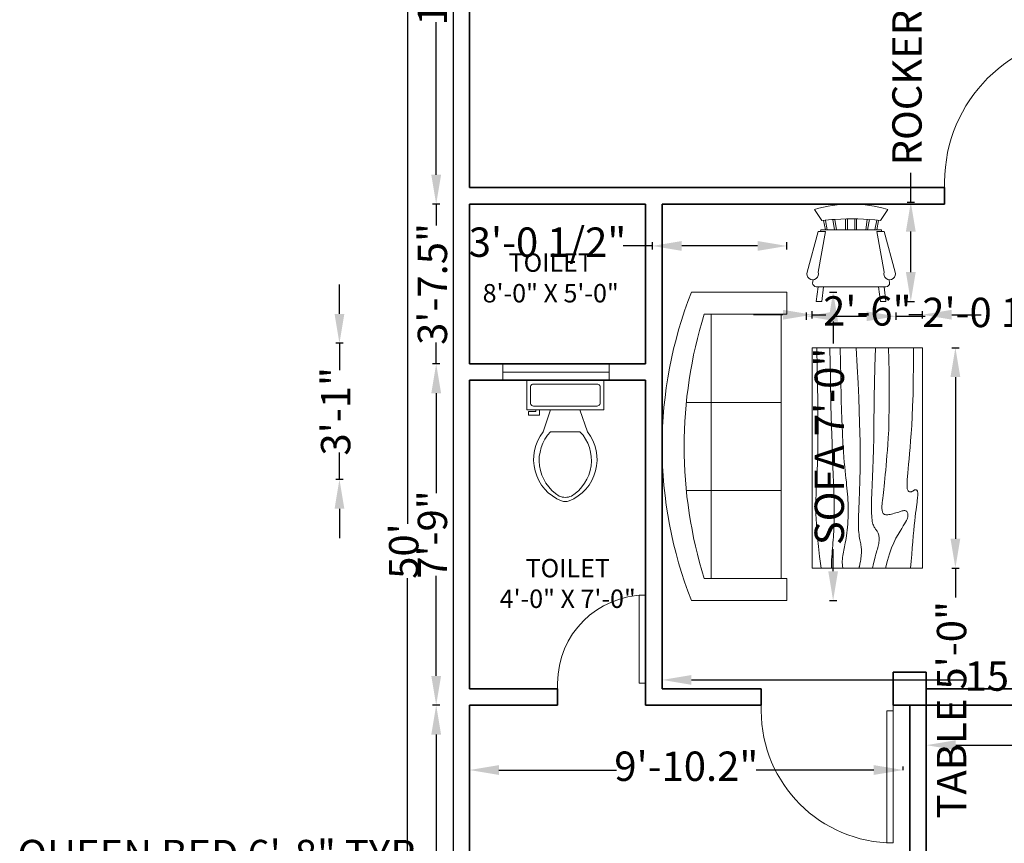
# Model space of a CAD drawing. Units: inches. Extents: x 2174 to 2692, y 577 to 1264.
# Tile 2 of 5: x 2174 to 2442, y 841 to 1065. Entities that reach past the tile are written whole.
import ezdxf

# ---------------------------------------------------------------- set-up
doc = ezdxf.new("R2010")
doc.units = ezdxf.units.IN
for name, color, linetype, lineweight in [('A-ANNO-DIMS', 2, 'Continuous', 13), ('A-AREA-IDEN', 7, 'Continuous', 18), ('A-COLS', 7, 'Continuous', 35), ('A-DOOR', 3, 'Continuous', 18), ('A-FLOR-FIXT', 9, 'Continuous', 18), ('A-FURN', 8, 'Continuous', 18), ('A-GLAZ', 4, 'Continuous', 18), ('A-WALL', 7, 'Continuous', 35), ('C-PROP', 7, 'Continuous', 25)]:
    doc.layers.add(name, color=color, linetype=linetype, lineweight=lineweight)
doc.styles.get("Standard").update_dxf_attribs({"font": 'arial.ttf'})
doc.dimstyles.new('ISO-25', dxfattribs={"dimtxt": 8, "dimasz": 8, "dimexe": 1, "dimexo": 1, "dimtad": 0, "dimdec": 1, "dimlunit": 3, "dimtxsty": 'Standard', "dimcen": 2.5, "dimclrd": 1, "dimclre": 1, "dimclrt": 1, "dimadec": 0, "dimazin": 0, "dimtfac": 1, "dimtdec": 1, "dimtmove": 0, "dimatfit": 3, "dimfxl": 1, "dimfxlon": 1, "dimarcsym": 0})

# ---------------------------------------------------------------- blocks, each defined once
blk = doc.blocks.new('Sofa - Roundback 7 ft.')
for p, q in [((-12.00002, -32.4421), (-12.00003, -6.5971)), ((11.99997, -32.4421), (11.99998, -6.5971)), ((-36.000027, -34), (-36.000027, -11.4696)), ((-35.999844, -13.3819), (35.9998, -13.3819)), ((35.99998, -34), (35.99998, -11.4696)), ((-36.000027, -32.4421), (35.99998, -32.4421))]:
    blk.add_line(p, q)
for points in [[(-36.000027, -34), (-42.000027, -34), (-42.000027, -8)], [(41.99998, -8), (41.99998, -34), (35.99998, -34)]]:
    blk.add_lwpolyline(points)
for centre, radius, start, end in [((0, -114.25), 114.25, 68.43141, 111.5686), ((-0.00001, -127.1968), 121.1968, 72.72033, 107.2797)]:
    blk.add_arc(centre, radius, start, end)
blk = doc.blocks.new('Chair - Rocking')
for p, q in [((-8, -4.5), (-10, -1.5)), ((8, -4.5), (10, -1.5)), ((-7.5, -4.5), (-7, -7)), ((-6.5, -7), (-7.02225, -4.43)), ((-4.5, -7), (-4.96674, -4.19951)), ((-4, -7), (-4.40532, -4.16272)), ((-1.5, -4.05012), (-1.5, -7)), ((-1, -7), (-1, -4.05012)), ((1, -7), (1, -4.04655)), ((1.5, -4.05012), (1.5, -7)), ((4, -7), (4.40187, -4.18694)), ((4.5, -7), (4.96761, -4.19437)), ((6.5, -7), (7, -4.4057)), ((7.5, -4.5), (7, -7)), ((-9, -7.5), (-12, -18.49999)), ((-7, -7.5), (-9, -7.5)), ((-9, -18.49999), (-7, -7.5)), ((-8.23428, -6.99939), (-8.3093, -7.47958)), ((-8.23041, -7), (8.23915, -7)), ((7, -7.5), (9, -7.5)), ((9, -18.49999), (7, -7.5)), ((8.31071, -7.48854), (8.23449, -7.00073)), ((9, -7.5), (12, -18.49999)), ((-10.36644, -20.64523), (-10.5, -21.49999)), ((10.5, -21.49999), (10.3575, -20.58798)), ((-9, -22.49999), (-9.5, -26.49999)), ((0, -22.49999), (-9.5, -22.49999)), ((-8, -26.49999), (-7.5, -22.49999)), ((0, -22.49999), (9.5, -22.49999)), ((8, -26.49999), (7.5, -22.49999)), ((9, -22.49999), (9.5, -26.49999)), ((-9.5, -26.49999), (-8, -26.49999)), ((9.5, -26.49999), (8, -26.49999))]:
    blk.add_line(p, q)
for centre, radius, start, end in [((0, -34.08333), 34.08333, 72.93847, 107.0615), ((0, -68.25004), 64.25, 93.92211, 97.15267), ((0, -68.25004), 64.25, 82.84733, 93.92211), ((-10.5, -18.99999), 1.58114, 161.5651, 18.43495), ((10.5, -18.99999), 1.58114, 161.5651, 18.43495), ((-9.5, -21.49999), 1, 180, 270), ((9.5, -21.49999), 1, 270, 0)]:
    blk.add_arc(centre, radius, start, end)
blk = doc.blocks.new('Toilet - top')
for p, q in [((9.5, -6), (9.5, -2)), ((-8, -8.5), (-8, -8)), ((-7, -8), (-7, -9.5)), ((-4, -8), (-6, -14)), ((4, -8), (6, -14)), ((-10, -8.5), (-8, -8.5)), ((-10, -9.5), (-10, -8.5)), ((-7, -9.5), (-10, -9.5)), ((4, -14), (-4, -14))]:
    blk.add_line(p, q)
blk.add_lwpolyline([(10.5, -8), (10.5, 0), (-10.5, 0), (-10.5, -8)], close=True)
for points in [[(-9.5, -2), (-9.5, -6)], [(8.5, -1), (-8.5, -1)], [(-8.5, -7), (8.5, -7)]]:
    blk.add_lwpolyline(points)
for centre, radius, start, end in [((-8.62, -1.88), 0.884, 81.8699, 188.1301), ((8.62, -1.88), 0.884, 351.8699, 98.1301), ((-8.62, -6.12), 0.884, 171.8699, 278.1301), ((8.62, -6.12), 0.884, 261.8699, 8.1301), ((3.52, -21.58), 12.17, 141.4691, 247.9714), ((4.2, -21.82), 11.33, 136.3677, 238.9468), ((-3.52, -21.58), 12.17, 292.0284, 38.5307), ((-4.2, -21.82), 11.33, 301.053, 43.6321), ((0, -27.88), 4, 245.7318, 294.2682), ((0, -29), 4, 254.8605, 285.1395)]:
    blk.add_arc(centre, radius, start, end)
blk = doc.blocks.new('Table - Rectangular Woodgrain 60 x 30 in.')
for p, q in [((0, 0), (0, -30)), ((60, 0), (0, 0)), ((60, -30), (60, 0)), ((0, -30), (60, -30))]:
    blk.add_line(p, q)
for points in [[(0, -2.4), (4.8155, -2.418), (9.0302, -2.4688), (12.709, -2.5477), (15.9167, -2.65), (18.7181, -2.7711), (21.1781, -2.9063), (23.3616, -3.0508), (25.3333, -3.2), (27.1477, -3.3495), (28.8172, -3.4958), (30.3437, -3.636), (31.7291, -3.7667), (32.9756, -3.8849), (34.0849, -3.9875), (35.059, -4.0714), (35.9, -4.1334), (36.6114, -4.1711), (37.2041, -4.1854), (37.6906, -4.1779), (38.0833, -4.15), (38.3948, -4.1034), (38.6375, -4.0396), (38.8239, -3.9602), (38.9666, -3.8667), (39.0764, -3.7608), (39.1573, -3.6448), (39.2116, -3.521), (39.2416, -3.3917), (39.2498, -3.2593), (39.2385, -3.1261), (39.21, -2.9944), (39.1666, -2.8667), (39.111, -2.7447), (39.0468, -2.6281), (38.978, -2.5163), (38.9083, -2.4083), (38.8418, -2.3035), (38.7823, -2.201), (38.7337, -2.1001), (38.7, -2), (38.6844, -1.9003), (38.6875, -1.8021), (38.7094, -1.707), (38.75, -1.6167), (38.8094, -1.5326), (38.8875, -1.4563), (38.9844, -1.3893), (39.1, -1.3333), (39.2351, -1.2896), (39.3937, -1.2583), (39.5804, -1.2396), (39.8, -1.2333), (40.057, -1.2396), (40.3562, -1.2583), (40.7023, -1.2896), (41.1, -1.3333), (41.5547, -1.3895), (42.0755, -1.4573), (42.6721, -1.5361), (43.3542, -1.625), (44.1316, -1.7233), (45.014, -1.8302), (46.0114, -1.9449), (47.1333, -2.0667), (48.3862, -2.1947), (49.7625, -2.3281), (51.2513, -2.4663), (52.8416, -2.6083), (54.5226, -2.7535), (56.2833, -2.9011), (58.1127, -3.0501), (60, -3.2)], [(0, -9.2), (6.5759, -9.0858), (11.9385, -9.0365), (16.2527, -9.0418), (19.6833, -9.0917), (22.3952, -9.1759), (24.5531, -9.2844), (26.322, -9.4069), (27.8666, -9.5333), (29.3241, -9.6553), (30.7203, -9.7719), (32.0532, -9.8837), (33.3208, -9.9917), (34.5213, -10.0965), (35.6526, -10.199), (36.7128, -10.2999), (37.7, -10.4), (38.6129, -10.4996), (39.4531, -10.5969), (40.223, -10.6895), (40.925, -10.775), (41.5613, -10.8512), (42.1344, -10.9156), (42.6465, -10.966), (43.1, -11), (43.4976, -11.0158), (43.8437, -11.0136), (44.143, -10.9942), (44.4, -10.9583), (44.6195, -10.9069), (44.8062, -10.8406), (44.9648, -10.7603), (45.1, -10.6667), (45.2155, -10.5598), (45.3114, -10.4365), (45.3871, -10.2929), (45.4416, -10.125), (45.4743, -9.929), (45.4844, -9.7011), (45.4709, -9.4371), (45.4333, -9.1333), (45.3716, -8.7883), (45.2896, -8.4104), (45.1919, -8.0107), (45.0833, -7.6), (44.9685, -7.1893), (44.8521, -6.7896), (44.7388, -6.4117), (44.6333, -6.0667), (44.54, -5.7628), (44.4614, -5.4979), (44.4001, -5.2675), (44.3583, -5.0667), (44.3384, -4.8909), (44.3427, -4.7354), (44.3736, -4.5956), (44.4333, -4.4667), (44.5236, -4.3453), (44.6427, -4.2333), (44.7884, -4.1339), (44.9583, -4.05), (45.1501, -3.9849), (45.3614, -3.9417), (45.59, -3.9234), (45.8333, -3.9333), (46.0915, -3.9749), (46.3734, -4.0531), (46.6906, -4.1736), (47.0542, -4.3417), (47.4756, -4.5629), (47.9661, -4.8427), (48.5372, -5.1866), (49.2, -5.6), (49.9676, -6.0844), (50.8594, -6.625), (51.8965, -7.2031), (53.1, -7.8), (54.491, -8.3969), (56.0906, -8.975), (57.9199, -9.5156), (60, -10)], [(0, -12.8), (5.1847, -12.9322), (9.6213, -13.0323), (13.3963, -13.1059), (16.5958, -13.1583), (19.3063, -13.1952), (21.614, -13.2219), (23.6054, -13.2439), (25.3666, -13.2667), (26.9728, -13.2947), (28.4531, -13.3281), (29.8256, -13.3663), (31.1083, -13.4083), (32.3191, -13.4535), (33.476, -13.501), (34.597, -13.5501), (35.7, -13.6), (36.7984, -13.6497), (37.8875, -13.6979), (38.9578, -13.743), (40, -13.7833), (41.0047, -13.8174), (41.9625, -13.8438), (42.864, -13.8607), (43.7, -13.8667), (44.4631, -13.8604), (45.1552, -13.8417), (45.7801, -13.8104), (46.3416, -13.7667), (46.8439, -13.7104), (47.2906, -13.6417), (47.6858, -13.5604), (48.0333, -13.4667), (48.3375, -13.3608), (48.6042, -13.2448), (48.8396, -13.121), (49.05, -12.9917), (49.2417, -12.8593), (49.4208, -12.7261), (49.5937, -12.5944), (49.7667, -12.4667), (49.9452, -12.3451), (50.1323, -12.2313), (50.3303, -12.1268), (50.5416, -12.0333), (50.7686, -11.9524), (51.0135, -11.8854), (51.2788, -11.8341), (51.5666, -11.8), (51.8785, -11.7843), (52.2116, -11.7865), (52.562, -11.8059), (52.926, -11.8417), (53.2998, -11.8931), (53.6795, -11.9594), (54.0614, -12.0397), (54.4416, -12.1333), (54.8223, -12.2401), (55.2293, -12.3625), (55.6942, -12.5037), (56.2489, -12.6667), (56.9251, -12.8547), (57.7545, -13.0708), (58.7689, -13.3182), (60, -13.6)], [(0, -18), (5.124, -17.7273), (9.6609, -17.5057), (13.6705, -17.3303), (17.2125, -17.1958), (20.3467, -17.0973), (23.1328, -17.0297), (25.6307, -16.9878), (27.9, -16.9667), (29.9928, -16.9617), (31.9302, -16.9703), (33.7254, -16.9907), (35.3917, -17.0208), (36.9423, -17.0588), (38.3906, -17.1026), (39.7499, -17.1503), (41.0333, -17.2), (42.2519, -17.2496), (43.4073, -17.2969), (44.4986, -17.3395), (45.525, -17.375), (46.4858, -17.4012), (47.3802, -17.4156), (48.2074, -17.416), (48.9667, -17.4), (49.6583, -17.3662), (50.2872, -17.3167), (50.8595, -17.2547), (51.3812, -17.1833), (51.8584, -17.1057), (52.2971, -17.025), (52.7034, -16.9443), (53.0833, -16.8667), (53.443, -16.7951), (53.789, -16.7313), (54.128, -16.6768), (54.4666, -16.6334), (54.8115, -16.6024), (55.1693, -16.5854), (55.5465, -16.5841), (55.95, -16.6), (56.3828, -16.6337), (56.8346, -16.6823), (57.2915, -16.7418), (57.7396, -16.8084), (58.165, -16.878), (58.5539, -16.9469), (58.8924, -17.0111), (59.1666, -17.0667), (59.3679, -17.1107), (59.5078, -17.1438), (59.6032, -17.1675), (59.6708, -17.1833), (59.7275, -17.193), (59.7901, -17.1979), (59.8753, -17.1998), (60, -17.2)], [(0, -22.4), (8.0098, -22.2501), (14.4094, -22.1011), (19.4168, -21.9535), (23.25, -21.8083), (26.1269, -21.6663), (28.2656, -21.5281), (29.884, -21.3947), (31.2, -21.2667), (32.3967, -21.1448), (33.5172, -21.0292), (34.5697, -20.9198), (35.5625, -20.8167), (36.5037, -20.7198), (37.4015, -20.6292), (38.2642, -20.5448), (39.1, -20.4667), (39.9164, -20.3951), (40.7187, -20.3313), (41.5117, -20.2768), (42.3, -20.2333), (43.0883, -20.2024), (43.8812, -20.1854), (44.6836, -20.1841), (45.5, -20.2), (46.3328, -20.234), (47.1747, -20.2844), (48.0163, -20.3488), (48.8479, -20.425), (49.66, -20.5106), (50.4429, -20.6031), (51.1872, -20.7004), (51.8833, -20.8), (52.5246, -20.8999), (53.1166, -20.9995), (53.6681, -21.0983), (54.1875, -21.1958), (54.6834, -21.2919), (55.1646, -21.3859), (55.6394, -21.4777), (56.1167, -21.5667), (56.6028, -21.6515), (57.0961, -21.7266), (57.5929, -21.7852), (58.0896, -21.8208), (58.5823, -21.8268), (59.0674, -21.7964), (59.5412, -21.723), (60, -21.6)], [(0, -25.2), (8.6355, -25.0504), (15.7026, -24.9031), (21.4049, -24.7606), (25.9458, -24.625), (29.529, -24.4988), (32.3578, -24.3844), (34.6359, -24.284), (36.5667, -24.2), (38.3213, -24.1341), (39.9417, -24.0854), (41.437, -24.0523), (42.8167, -24.0333), (44.0901, -24.0268), (45.2667, -24.0313), (46.3557, -24.0451), (47.3667, -24.0667), (48.309, -24.0947), (49.1928, -24.1287), (50.0284, -24.168), (50.826, -24.2125), (51.5959, -24.2617), (52.3483, -24.3151), (53.0935, -24.3725), (53.8417, -24.4334), (54.6009, -24.497), (55.3699, -24.561), (56.1454, -24.6226), (56.9239, -24.6792), (57.7021, -24.7279), (58.4764, -24.7662), (59.2435, -24.7911), (60, -24.8)], [(0, -28.8), (5.6867, -28.6681), (10.45, -28.5698), (14.407, -28.5012), (17.675, -28.4584), (20.3711, -28.4374), (22.6125, -28.4344), (24.5164, -28.4455), (26.2, -28.4667), (27.762, -28.4947), (29.2276, -28.5281), (30.6033, -28.5663), (31.8958, -28.6084), (33.1118, -28.6535), (34.2578, -28.7011), (35.3405, -28.7501), (36.3666, -28.8), (37.3443, -28.8497), (38.288, -28.8974), (39.2137, -28.9412), (40.1375, -28.9792), (41.0753, -29.0093), (42.0432, -29.0297), (43.0572, -29.0384), (44.1333, -29.0333), (45.2936, -29.0114), (46.5843, -28.9641), (48.0579, -28.8816), (49.7666, -28.7542), (51.7629, -28.5721), (54.0989, -28.3255), (56.8272, -28.0048), (60, -27.6)]]:
    blk.add_lwpolyline(points)
blk = doc.blocks.new('*D12')
at = {"layer": 'A-ANNO-DIMS', "color": 0, "lineweight": -2, "transparency": 16777216}
for p, q in [((2348.95, 885.56), (2348.95, 884.25)), ((2356.95, 885.25), (2431.92, 885.25)), ((2520.95, 885.25), (2445.99, 885.25)), ((2528.95, 885.56), (2528.95, 884.25))]:
    blk.add_line(p, q, dxfattribs=at)
at = {"layer": 'A-ANNO-DIMS', "color": 0, "transparency": 16777216}
for points in [[(2356.95, 886.58), (2356.95, 883.91), (2348.95, 885.25)], [(2520.95, 886.58), (2520.95, 883.91), (2528.95, 885.25)]]:
    blk.add_solid(points, dxfattribs=at)
at = {"layer": 'Defpoints', "color": 0, "transparency": 16777216}
for p in [(2348.95, 886.56), (2528.95, 886.56), (2348.95, 885.25)]:
    blk.add_point(p, dxfattribs=at)
at = {"layer": 'A-ANNO-DIMS', "color": 0, "transparency": 16777216, "insert": (2438.95, 885.25), "char_height": 8, "attachment_point": 5}
blk.add_mtext("15'", dxfattribs=at)
blk = doc.blocks.new('*D13')
at = {"layer": 'A-ANNO-DIMS', "color": 0, "lineweight": -2, "transparency": 16777216}
for p, q in [((2420.95, 868.48), (2420.95, 866.48)), ((2428.95, 867.48), (2479.92, 867.48)), ((2544.95, 867.48), (2493.99, 867.48)), ((2552.95, 868.48), (2552.95, 866.48))]:
    blk.add_line(p, q, dxfattribs=at)
at = {"layer": 'A-ANNO-DIMS', "color": 0, "transparency": 16777216}
for points in [[(2428.95, 868.81), (2428.95, 866.15), (2420.95, 867.48)], [(2544.95, 868.81), (2544.95, 866.15), (2552.95, 867.48)]]:
    blk.add_solid(points, dxfattribs=at)
at = {"layer": 'Defpoints', "color": 0, "transparency": 16777216}
for p in [(2420.95, 878.35), (2552.95, 878.35), (2420.95, 867.48)]:
    blk.add_point(p, dxfattribs=at)
at = {"layer": 'A-ANNO-DIMS', "color": 0, "transparency": 16777216, "insert": (2486.95, 867.48), "char_height": 8, "attachment_point": 5}
blk.add_mtext("11'", dxfattribs=at)
blk = doc.blocks.new('*D14')
at = {"layer": 'A-ANNO-DIMS', "color": 0, "lineweight": -2, "transparency": 16777216}
for p, q in [((2296.45, 860.7), (2296.45, 861.7)), ((2414.64, 860.7), (2414.64, 861.7)), ((2304.45, 860.7), (2336.52, 860.7)), ((2406.64, 860.7), (2374.57, 860.7))]:
    blk.add_line(p, q, dxfattribs=at)
at = {"layer": 'A-ANNO-DIMS', "color": 0, "transparency": 16777216}
for points in [[(2304.45, 862.03), (2304.45, 859.37), (2296.45, 860.7)], [(2406.64, 862.03), (2406.64, 859.37), (2414.64, 860.7)]]:
    blk.add_solid(points, dxfattribs=at)
at = {"layer": 'Defpoints', "color": 0, "transparency": 16777216}
for p in [(2296.45, 860.7), (2414.64, 860.7), (2414.64, 860.7)]:
    blk.add_point(p, dxfattribs=at)
at = {"layer": 'A-ANNO-DIMS', "color": 0, "transparency": 16777216, "insert": (2355.54, 860.7), "char_height": 8, "attachment_point": 5}
blk.add_mtext('9\'-10.2"', dxfattribs=at)
blk = doc.blocks.new('*U25')
for p, q in [((-24, 0), (-24, -6)), ((0, 0), (0, -6))]:
    blk.add_line(p, q)
blk.add_lwpolyline([(0, 0), (0, 24), (-1.75, 24), (-1.75, 0)], close=True)
blk.add_arc((0, 0), 24, 90, 180)
blk = doc.blocks.new('*U24')
for p, q in [((0, 0), (0, -6)), ((-40, 0), (-40, -6))]:
    blk.add_line(p, q)
blk.add_lwpolyline([(0, 0), (0, 40), (-1.75, 40), (-1.75, 0)], close=True)
blk.add_arc((0, 0), 40, 90, 180)
blk = doc.blocks.new('*U26')
for p, q in [((-36, 0), (-36, 6)), ((0, 0), (0, 6))]:
    blk.add_line(p, q)
blk.add_lwpolyline([(0, 0), (0, -36), (-1.75, -36), (-1.75, 0)], close=True)
blk.add_arc((0, 0), 36, 180, 270)
blk = doc.blocks.new('*D30')
at = {"layer": 'A-ANNO-DIMS', "color": 0, "lineweight": -2, "transparency": 16777216}
for p, q in [((2288.37, 1151.35), (2286.37, 1151.35)), ((2287.37, 1143.35), (2287.37, 1101.75)), ((2287.37, 1022.85), (2287.37, 1064.45)), ((2288.37, 1014.85), (2286.37, 1014.85))]:
    blk.add_line(p, q, dxfattribs=at)
at = {"layer": 'A-ANNO-DIMS', "color": 0, "transparency": 16777216}
for points in [[(2286.03, 1143.35), (2288.7, 1143.35), (2287.37, 1151.35)], [(2286.03, 1022.85), (2288.7, 1022.85), (2287.37, 1014.85)]]:
    blk.add_solid(points, dxfattribs=at)
at = {"layer": 'Defpoints', "color": 0, "transparency": 16777216}
for p in [(2291.95, 1151.35), (2287.37, 1014.85), (2296.45, 1014.85)]:
    blk.add_point(p, dxfattribs=at)
at = {"layer": 'A-ANNO-DIMS', "color": 0, "transparency": 16777216, "insert": (2287.37, 1083.1), "char_height": 8, "attachment_point": 5, "rotation": 90}
blk.add_mtext('11\'-4.5"', dxfattribs=at)
blk = doc.blocks.new('*D31')
at = {"layer": 'A-ANNO-DIMS', "color": 0, "lineweight": -2, "transparency": 16777216}
for p, q in [((2287.37, 1022.85), (2287.37, 1030.85)), ((2288.37, 1014.85), (2286.37, 1014.85)), ((2287.37, 1014.85), (2287.37, 1009.02)), ((2287.37, 971.35), (2287.37, 977.19)), ((2288.37, 971.35), (2286.37, 971.35)), ((2287.37, 963.35), (2287.37, 955.35))]:
    blk.add_line(p, q, dxfattribs=at)
at = {"layer": 'A-ANNO-DIMS', "color": 0, "transparency": 16777216}
for points in [[(2286.03, 1022.85), (2288.7, 1022.85), (2287.37, 1014.85)], [(2286.03, 963.35), (2288.7, 963.35), (2287.37, 971.35)]]:
    blk.add_solid(points, dxfattribs=at)
at = {"layer": 'Defpoints', "color": 0, "transparency": 16777216}
for p in [(2296.45, 1014.85), (2287.37, 971.35), (2296.45, 971.35)]:
    blk.add_point(p, dxfattribs=at)
at = {"layer": 'A-ANNO-DIMS', "color": 0, "transparency": 16777216, "insert": (2287.37, 993.1), "char_height": 8, "attachment_point": 5, "rotation": 90}
blk.add_mtext('3\'-7.5"', dxfattribs=at)
blk = doc.blocks.new('*D32')
at = {"layer": 'A-ANNO-DIMS', "color": 0, "lineweight": -2, "transparency": 16777216}
for p, q in [((2288.37, 971.35), (2286.37, 971.35)), ((2287.37, 963.35), (2287.37, 936.08)), ((2287.37, 886.35), (2287.37, 913.63)), ((2288.37, 878.35), (2286.37, 878.35))]:
    blk.add_line(p, q, dxfattribs=at)
at = {"layer": 'A-ANNO-DIMS', "color": 0, "transparency": 16777216}
for points in [[(2286.03, 963.35), (2288.7, 963.35), (2287.37, 971.35)], [(2286.03, 886.35), (2288.7, 886.35), (2287.37, 878.35)]]:
    blk.add_solid(points, dxfattribs=at)
at = {"layer": 'Defpoints', "color": 0, "transparency": 16777216}
for p in [(2296.45, 971.35), (2287.37, 878.35), (2296.45, 878.35)]:
    blk.add_point(p, dxfattribs=at)
at = {"layer": 'A-ANNO-DIMS', "color": 0, "transparency": 16777216, "insert": (2287.37, 924.85), "char_height": 8, "attachment_point": 5, "rotation": 90}
blk.add_mtext('7\'-9"', dxfattribs=at)
blk = doc.blocks.new('*D33')
at = {"layer": 'A-ANNO-DIMS', "color": 0, "lineweight": -2, "transparency": 16777216}
for p, q in [((2288.37, 878.35), (2286.37, 878.35)), ((2287.37, 870.35), (2287.37, 810.75)), ((2287.37, 713.85), (2287.37, 773.45)), ((2288.37, 705.85), (2286.37, 705.85))]:
    blk.add_line(p, q, dxfattribs=at)
at = {"layer": 'A-ANNO-DIMS', "color": 0, "transparency": 16777216}
for points in [[(2286.03, 870.35), (2288.7, 870.35), (2287.37, 878.35)], [(2286.03, 713.85), (2288.7, 713.85), (2287.37, 705.85)]]:
    blk.add_solid(points, dxfattribs=at)
at = {"layer": 'Defpoints', "color": 0, "transparency": 16777216}
for p in [(2296.45, 878.35), (2287.37, 705.85), (2296.45, 705.85)]:
    blk.add_point(p, dxfattribs=at)
at = {"layer": 'A-ANNO-DIMS', "color": 0, "transparency": 16777216, "insert": (2287.37, 792.1), "char_height": 8, "attachment_point": 5, "rotation": 90}
blk.add_mtext('14\'-4.5"', dxfattribs=at)
blk = doc.blocks.new('*D43')
at = {"layer": 'A-ANNO-DIMS', "color": 0, "lineweight": -2, "transparency": 16777216}
for p, q in [((2280.55, 1220.35), (2278.55, 1220.35)), ((2279.55, 1212.35), (2279.55, 927.77)), ((2279.55, 628.35), (2279.55, 912.94)), ((2280.55, 620.35), (2278.55, 620.35))]:
    blk.add_line(p, q, dxfattribs=at)
at = {"layer": 'A-ANNO-DIMS', "color": 0, "transparency": 16777216}
for points in [[(2278.21, 1212.35), (2280.88, 1212.35), (2279.55, 1220.35)], [(2278.21, 628.35), (2280.88, 628.35), (2279.55, 620.35)]]:
    blk.add_solid(points, dxfattribs=at)
at = {"layer": 'Defpoints', "color": 0, "transparency": 16777216}
for p in [(2291.95, 1220.35), (2279.55, 620.35), (2291.95, 620.35)]:
    blk.add_point(p, dxfattribs=at)
at = {"layer": 'A-ANNO-DIMS', "color": 0, "transparency": 16777216, "insert": (2279.55, 920.35), "char_height": 8, "attachment_point": 5, "rotation": 90}
blk.add_mtext("50'", dxfattribs=at)
blk = doc.blocks.new('*D45')
at = {"layer": 'A-ANNO-DIMS', "color": 1, "lineweight": -2, "transparency": 16777216}
for p, q in [((2296.45, 835.64), (2296.45, 837.64)), ((2376.45, 835.64), (2376.45, 837.64)), ((2296.45, 836.64), (2288.45, 836.64)), ((2368.45, 836.64), (2304.45, 836.64))]:
    blk.add_line(p, q, dxfattribs=at)
at = {"layer": 'A-ANNO-DIMS', "color": 1, "transparency": 16777216}
for points in [[(2304.45, 837.97), (2304.45, 835.3), (2296.45, 836.64)], [(2368.45, 837.97), (2368.45, 835.3), (2376.45, 836.64)]]:
    blk.add_solid(points, dxfattribs=at)
at = {"layer": 'Defpoints', "color": 0, "transparency": 16777216}
for p in [(2296.45, 836.64), (2296.45, 824.64), (2376.45, 824.64)]:
    blk.add_point(p, dxfattribs=at)
at = {"layer": 'A-ANNO-DIMS', "color": 1, "transparency": 16777216, "insert": (2228.99, 836.64), "char_height": 8, "attachment_point": 5}
blk.add_mtext('QUEEN BED 6\'-8" TYP.', dxfattribs=at)
blk = doc.blocks.new('*D51')
at = {"layer": 'A-ANNO-DIMS', "color": 1, "lineweight": -2, "transparency": 16777216}
for p, q in [((2394.55, 990.85), (2396.55, 990.85)), ((2395.55, 982.85), (2395.55, 976.86)), ((2395.55, 914.85), (2395.55, 920.85)), ((2394.55, 906.85), (2396.55, 906.85))]:
    blk.add_line(p, q, dxfattribs=at)
at = {"layer": 'A-ANNO-DIMS', "color": 1, "transparency": 16777216}
for points in [[(2394.22, 982.85), (2396.89, 982.85), (2395.55, 990.85)], [(2394.22, 914.85), (2396.89, 914.85), (2395.55, 906.85)]]:
    blk.add_solid(points, dxfattribs=at)
at = {"layer": 'Defpoints', "color": 0, "transparency": 16777216}
for p in [(2382.95, 990.85), (2395.55, 990.85), (2382.95, 906.85)]:
    blk.add_point(p, dxfattribs=at)
at = {"layer": 'A-ANNO-DIMS', "color": 1, "transparency": 16777216, "insert": (2395.55, 948.85), "char_height": 8, "attachment_point": 5, "rotation": 90}
blk.add_mtext('SOFA 7\'-0"', dxfattribs=at)
blk = doc.blocks.new('*D52')
at = {"layer": 'A-ANNO-DIMS', "color": 1, "lineweight": -2, "transparency": 16777216}
for p, q in [((2346.29, 1002.45), (2346.29, 1004.45)), ((2382.95, 1002.45), (2382.95, 1004.45)), ((2346.29, 1003.45), (2338.29, 1003.45)), ((2374.95, 1003.45), (2354.29, 1003.45))]:
    blk.add_line(p, q, dxfattribs=at)
at = {"layer": 'A-ANNO-DIMS', "color": 1, "transparency": 16777216}
for points in [[(2354.29, 1004.79), (2354.29, 1002.12), (2346.29, 1003.45)], [(2374.95, 1004.79), (2374.95, 1002.12), (2382.95, 1003.45)]]:
    blk.add_solid(points, dxfattribs=at)
at = {"layer": 'Defpoints', "color": 0, "transparency": 16777216}
for p in [(2346.29, 1003.45), (2346.29, 990.85), (2382.95, 990.85)]:
    blk.add_point(p, dxfattribs=at)
at = {"layer": 'A-ANNO-DIMS', "color": 1, "transparency": 16777216, "insert": (2317.71, 1003.45), "char_height": 8, "attachment_point": 5}
blk.add_mtext('3\'-0 1/2"', dxfattribs=at)
blk = doc.blocks.new('*D53')
at = {"layer": 'A-ANNO-DIMS', "color": 1, "lineweight": -2, "transparency": 16777216}
for p, q in [((2416.72, 1015.35), (2416.72, 1023.35)), ((2415.72, 1015.35), (2417.72, 1015.35)), ((2416.72, 996.35), (2416.72, 1007.35)), ((2415.72, 988.35), (2417.72, 988.35))]:
    blk.add_line(p, q, dxfattribs=at)
at = {"layer": 'A-ANNO-DIMS', "color": 1, "transparency": 16777216}
for points in [[(2415.39, 1007.35), (2418.06, 1007.35), (2416.72, 1015.35)], [(2415.39, 996.35), (2418.06, 996.35), (2416.72, 988.35)]]:
    blk.add_solid(points, dxfattribs=at)
at = {"layer": 'Defpoints', "color": 0, "transparency": 16777216}
for p in [(2412.67, 1015.35), (2416.72, 1015.35), (2412.67, 988.35)]:
    blk.add_point(p, dxfattribs=at)
at = {"layer": 'A-ANNO-DIMS', "color": 1, "transparency": 16777216, "insert": (2416.72, 1059.86), "char_height": 8, "attachment_point": 5, "rotation": 90}
blk.add_mtext('ROCKER 2\'-3"', dxfattribs=at)
blk = doc.blocks.new('*D54')
at = {"layer": 'A-ANNO-DIMS', "color": 1, "lineweight": -2, "transparency": 16777216}
for p, q in [((2388.24, 985.3), (2388.24, 983.3)), ((2412.67, 985.3), (2412.67, 983.3)), ((2396.24, 984.3), (2404.67, 984.3)), ((2412.67, 984.3), (2420.67, 984.3))]:
    blk.add_line(p, q, dxfattribs=at)
at = {"layer": 'A-ANNO-DIMS', "color": 1, "transparency": 16777216}
for points in [[(2396.24, 985.64), (2396.24, 982.97), (2388.24, 984.3)], [(2404.67, 985.64), (2404.67, 982.97), (2412.67, 984.3)]]:
    blk.add_solid(points, dxfattribs=at)
at = {"layer": 'Defpoints', "color": 0, "transparency": 16777216}
for p in [(2388.24, 988.35), (2412.67, 988.35), (2412.67, 984.3)]:
    blk.add_point(p, dxfattribs=at)
at = {"layer": 'A-ANNO-DIMS', "color": 1, "transparency": 16777216, "insert": (2441.32, 984.3), "char_height": 8, "attachment_point": 5}
blk.add_mtext('2\'-0 1/2"', dxfattribs=at)
blk = doc.blocks.new('*D61')
at = {"layer": 'A-ANNO-DIMS', "color": 1, "lineweight": -2, "transparency": 16777216}
for p, q in [((2427.87, 975.72), (2429.87, 975.72)), ((2428.87, 967.72), (2428.87, 923.72)), ((2427.87, 915.72), (2429.87, 915.72)), ((2428.87, 915.72), (2428.87, 907.72))]:
    blk.add_line(p, q, dxfattribs=at)
at = {"layer": 'A-ANNO-DIMS', "color": 1, "transparency": 16777216}
for points in [[(2427.54, 967.72), (2430.21, 967.72), (2428.87, 975.72)], [(2427.54, 923.72), (2430.21, 923.72), (2428.87, 915.72)]]:
    blk.add_solid(points, dxfattribs=at)
at = {"layer": 'Defpoints', "color": 0, "transparency": 16777216}
for p in [(2419.87, 975.72), (2419.87, 915.72), (2428.87, 915.72)]:
    blk.add_point(p, dxfattribs=at)
at = {"layer": 'A-ANNO-DIMS', "color": 1, "transparency": 16777216, "insert": (2428.87, 877.1), "char_height": 8, "attachment_point": 5, "rotation": 90}
blk.add_mtext('TABLE 5\'-0"', dxfattribs=at)
blk = doc.blocks.new('*D62')
at = {"layer": 'A-ANNO-DIMS', "color": 1, "lineweight": -2, "transparency": 16777216}
for p, q in [((2389.87, 983.72), (2389.87, 985.72)), ((2419.87, 983.72), (2419.87, 985.72)), ((2381.87, 984.72), (2373.87, 984.72)), ((2389.87, 984.72), (2393.55, 984.72)), ((2419.87, 984.72), (2416.2, 984.72)), ((2427.87, 984.72), (2435.87, 984.72))]:
    blk.add_line(p, q, dxfattribs=at)
at = {"layer": 'A-ANNO-DIMS', "color": 1, "transparency": 16777216}
for points in [[(2381.87, 986.05), (2381.87, 983.38), (2389.87, 984.72)], [(2427.87, 986.05), (2427.87, 983.38), (2419.87, 984.72)]]:
    blk.add_solid(points, dxfattribs=at)
at = {"layer": 'Defpoints', "color": 0, "transparency": 16777216}
for p in [(2419.87, 984.72), (2389.87, 975.72), (2419.87, 975.72)]:
    blk.add_point(p, dxfattribs=at)
at = {"layer": 'A-ANNO-DIMS', "color": 1, "transparency": 16777216, "insert": (2404.87, 984.72), "char_height": 8, "attachment_point": 5}
blk.add_mtext('2\'-6"', dxfattribs=at)
blk = doc.blocks.new('*D63')
at = {"layer": 'A-ANNO-DIMS', "color": 1, "lineweight": -2, "transparency": 16777216}
for p, q in [((2360.45, 590.4), (2360.45, 588.4)), ((2392.45, 590.4), (2392.45, 588.4)), ((2352.45, 589.4), (2344.45, 589.4)), ((2360.45, 589.4), (2365.13, 589.4)), ((2392.45, 589.4), (2387.78, 589.4)), ((2400.45, 589.4), (2408.45, 589.4))]:
    blk.add_line(p, q, dxfattribs=at)
at = {"layer": 'A-ANNO-DIMS', "color": 1, "transparency": 16777216}
for points in [[(2352.45, 590.74), (2352.45, 588.07), (2360.45, 589.4)], [(2400.45, 590.74), (2400.45, 588.07), (2392.45, 589.4)]]:
    blk.add_solid(points, dxfattribs=at)
at = {"layer": 'Defpoints', "color": 0, "transparency": 16777216}
for p in [(2360.45, 1155.85), (2392.45, 1155.6), (2392.45, 589.4)]:
    blk.add_point(p, dxfattribs=at)
at = {"layer": 'A-ANNO-DIMS', "color": 1, "transparency": 16777216, "insert": (2376.45, 589.4), "char_height": 8, "attachment_point": 5}
blk.add_mtext('2\'-8"', dxfattribs=at)
blk = doc.blocks.new('*D65')
at = {"layer": 'A-ANNO-DIMS', "color": 1, "lineweight": -2, "transparency": 16777216}
for p, q in [((2412.95, 1251.3), (2404.95, 1251.3)), ((2420.95, 1250.3), (2420.95, 1252.3)), ((2420.95, 1251.3), (2423.52, 1251.3)), ((2454.95, 1251.3), (2452.39, 1251.3)), ((2454.95, 1250.3), (2454.95, 1252.3)), ((2462.95, 1251.3), (2470.95, 1251.3))]:
    blk.add_line(p, q, dxfattribs=at)
at = {"layer": 'A-ANNO-DIMS', "color": 1, "transparency": 16777216}
for points in [[(2412.95, 1252.64), (2412.95, 1249.97), (2420.95, 1251.3)], [(2462.95, 1252.64), (2462.95, 1249.97), (2454.95, 1251.3)]]:
    blk.add_solid(points, dxfattribs=at)
at = {"layer": 'Defpoints', "color": 0, "transparency": 16777216}
for p in [(2454.95, 1251.3), (2420.95, 698.35), (2454.95, 698.35)]:
    blk.add_point(p, dxfattribs=at)
at = {"layer": 'A-ANNO-DIMS', "color": 1, "transparency": 16777216, "insert": (2437.95, 1251.3), "char_height": 8, "attachment_point": 5}
blk.add_mtext('2\'-10"', dxfattribs=at)
blk = doc.blocks.new('*D67')
at = {"layer": 'A-ANNO-DIMS', "color": 1, "lineweight": -2, "transparency": 16777216}
for p, q in [((2312.45, 1251.3), (2304.45, 1251.3)), ((2320.45, 1250.3), (2320.45, 1252.3)), ((2320.45, 1251.3), (2321.13, 1251.3)), ((2344.45, 1251.3), (2343.78, 1251.3)), ((2344.45, 1250.3), (2344.45, 1252.3)), ((2352.45, 1251.3), (2360.45, 1251.3))]:
    blk.add_line(p, q, dxfattribs=at)
at = {"layer": 'A-ANNO-DIMS', "color": 1, "transparency": 16777216}
for points in [[(2312.45, 1252.64), (2312.45, 1249.97), (2320.45, 1251.3)], [(2352.45, 1252.64), (2352.45, 1249.97), (2344.45, 1251.3)]]:
    blk.add_solid(points, dxfattribs=at)
at = {"layer": 'Defpoints', "color": 0, "transparency": 16777216}
for p in [(2344.45, 1251.3), (2320.45, 882.85), (2344.45, 882.85)]:
    blk.add_point(p, dxfattribs=at)
at = {"layer": 'A-ANNO-DIMS', "color": 1, "transparency": 16777216, "insert": (2332.45, 1251.3), "char_height": 8, "attachment_point": 5}
blk.add_mtext('2\'-0"', dxfattribs=at)
blk = doc.blocks.new('*D68')
at = {"layer": 'A-ANNO-DIMS', "color": 1, "lineweight": -2, "transparency": 16777216}
for p, q in [((2367.95, 1251.3), (2359.95, 1251.3)), ((2375.95, 1250.3), (2375.95, 1252.3)), ((2375.95, 1251.3), (2382.7, 1251.3)), ((2411.95, 1251.3), (2405.21, 1251.3)), ((2411.95, 1250.3), (2411.95, 1252.3)), ((2419.95, 1251.3), (2427.95, 1251.3))]:
    blk.add_line(p, q, dxfattribs=at)
at = {"layer": 'A-ANNO-DIMS', "color": 1, "transparency": 16777216}
for points in [[(2367.95, 1252.64), (2367.95, 1249.97), (2375.95, 1251.3)], [(2419.95, 1252.64), (2419.95, 1249.97), (2411.95, 1251.3)]]:
    blk.add_solid(points, dxfattribs=at)
at = {"layer": 'Defpoints', "color": 0, "transparency": 16777216}
for p in [(2411.95, 1251.3), (2375.95, 878.35), (2411.95, 878.35)]:
    blk.add_point(p, dxfattribs=at)
at = {"layer": 'A-ANNO-DIMS', "color": 1, "transparency": 16777216, "insert": (2393.95, 1251.3), "char_height": 8, "attachment_point": 5}
blk.add_mtext('3\'-0"', dxfattribs=at)
blk = doc.blocks.new('*D70')
at = {"layer": 'A-ANNO-DIMS', "color": 1, "lineweight": -2, "transparency": 16777216}
for p, q in [((2261, 984.94), (2261, 992.94)), ((2262, 976.94), (2260, 976.94)), ((2261, 976.94), (2261, 969.66)), ((2261, 939.87), (2261, 947.15)), ((2262, 939.87), (2260, 939.87)), ((2261, 931.87), (2261, 923.87))]:
    blk.add_line(p, q, dxfattribs=at)
at = {"layer": 'A-ANNO-DIMS', "color": 1, "transparency": 16777216}
for points in [[(2259.67, 984.94), (2262.34, 984.94), (2261, 976.94)], [(2259.67, 931.87), (2262.34, 931.87), (2261, 939.87)]]:
    blk.add_solid(points, dxfattribs=at)
at = {"layer": 'Defpoints', "color": 0, "transparency": 16777216}
for p in [(2528.95, 976.94), (2261, 939.87), (2528.95, 939.87)]:
    blk.add_point(p, dxfattribs=at)
at = {"layer": 'A-ANNO-DIMS', "color": 1, "transparency": 16777216, "insert": (2261, 958.41), "char_height": 8, "attachment_point": 5, "rotation": 90}
blk.add_mtext('3\'-1"', dxfattribs=at)
blk = doc.blocks.new('*D71')
at = {"layer": 'A-ANNO-DIMS', "color": 1, "lineweight": -2, "transparency": 16777216}
for p, q in [((2308.69, 1251.3), (2300.69, 1251.3)), ((2316.69, 1250.3), (2316.69, 1252.3)), ((2316.69, 1251.3), (2321.61, 1251.3)), ((2368.01, 1251.3), (2363.09, 1251.3)), ((2368.01, 1250.3), (2368.01, 1252.3)), ((2376.01, 1251.3), (2384.01, 1251.3))]:
    blk.add_line(p, q, dxfattribs=at)
at = {"layer": 'A-ANNO-DIMS', "color": 1, "transparency": 16777216}
for points in [[(2308.69, 1252.64), (2308.69, 1249.97), (2316.69, 1251.3)], [(2376.01, 1252.64), (2376.01, 1249.97), (2368.01, 1251.3)]]:
    blk.add_solid(points, dxfattribs=at)
at = {"layer": 'Defpoints', "color": 0, "transparency": 16777216}
for p in [(2368.01, 1251.3), (2316.69, 710.35), (2368.01, 710.35)]:
    blk.add_point(p, dxfattribs=at)
at = {"layer": 'A-ANNO-DIMS', "color": 1, "transparency": 16777216, "insert": (2342.35, 1251.3), "char_height": 8, "attachment_point": 5}
blk.add_mtext('4\'-3 1/2"', dxfattribs=at)
blk = doc.blocks.new('*D72')
at = {"layer": 'A-ANNO-DIMS', "color": 1, "lineweight": -2, "transparency": 16777216}
for p, q in [((2296.45, 1250.3), (2296.45, 1252.3)), ((2304.45, 1251.3), (2308.69, 1251.3)), ((2316.69, 1250.3), (2316.69, 1252.3)), ((2316.69, 1251.3), (2324.69, 1251.3))]:
    blk.add_line(p, q, dxfattribs=at)
at = {"layer": 'A-ANNO-DIMS', "color": 1, "transparency": 16777216}
for points in [[(2304.45, 1252.64), (2304.45, 1249.97), (2296.45, 1251.3)], [(2308.69, 1252.64), (2308.69, 1249.97), (2316.69, 1251.3)]]:
    blk.add_solid(points, dxfattribs=at)
at = {"layer": 'Defpoints', "color": 0, "transparency": 16777216}
for p in [(2316.69, 1251.3), (2296.45, 710.35), (2316.69, 710.35)]:
    blk.add_point(p, dxfattribs=at)
at = {"layer": 'A-ANNO-DIMS', "color": 1, "transparency": 16777216, "insert": (2335.57, 1251.3), "char_height": 8, "attachment_point": 5}
blk.add_mtext('1\'-8"', dxfattribs=at)
blk = doc.blocks.new('*D75')
at = {"layer": 'A-ANNO-DIMS', "color": 1, "lineweight": -2, "transparency": 16777216}
for p, q in [((2296.45, 590.4), (2296.45, 588.4)), ((2344.45, 590.4), (2344.45, 588.4)), ((2304.45, 589.4), (2309.03, 589.4)), ((2336.45, 589.4), (2331.87, 589.4))]:
    blk.add_line(p, q, dxfattribs=at)
at = {"layer": 'A-ANNO-DIMS', "color": 1, "transparency": 16777216}
for points in [[(2304.45, 590.74), (2304.45, 588.07), (2296.45, 589.4)], [(2336.45, 590.74), (2336.45, 588.07), (2344.45, 589.4)]]:
    blk.add_solid(points, dxfattribs=at)
at = {"layer": 'Defpoints', "color": 0, "transparency": 16777216}
for p in [(2296.45, 1014.85), (2344.45, 1014.85), (2344.45, 589.4)]:
    blk.add_point(p, dxfattribs=at)
at = {"layer": 'A-ANNO-DIMS', "color": 1, "transparency": 16777216, "insert": (2320.45, 589.4), "char_height": 8, "attachment_point": 5}
blk.add_mtext('4\'-0"', dxfattribs=at)
blk = doc.blocks.new('*D78')
at = {"layer": 'A-ANNO-DIMS', "color": 1, "lineweight": -2, "transparency": 16777216}
for p, q in [((2399.49, 590.4), (2399.49, 588.4)), ((2432.76, 590.4), (2432.76, 588.4)), ((2407.49, 589.4), (2424.76, 589.4)), ((2432.76, 589.4), (2440.76, 589.4))]:
    blk.add_line(p, q, dxfattribs=at)
at = {"layer": 'A-ANNO-DIMS', "color": 1, "transparency": 16777216}
for points in [[(2407.49, 590.74), (2407.49, 588.07), (2399.49, 589.4)], [(2424.76, 590.74), (2424.76, 588.07), (2432.76, 589.4)]]:
    blk.add_solid(points, dxfattribs=at)
at = {"layer": 'Defpoints', "color": 0, "transparency": 16777216}
for p in [(2399.49, 1151.35), (2432.76, 1151.35), (2432.76, 589.4)]:
    blk.add_point(p, dxfattribs=at)
at = {"layer": 'A-ANNO-DIMS', "color": 1, "transparency": 16777216, "insert": (2461.41, 589.4), "char_height": 8, "attachment_point": 5}
blk.add_mtext('2\'-9 1/2"', dxfattribs=at)

msp = doc.modelspace()

# ---------------------------------------------------------------- linework, layer by layer
at = {"layer": 'A-COLS'}
for p, q in [((2420.95, 887.35), (2411.95, 887.35)), ((2411.95, 887.35), (2411.95, 878.35)), ((2420.95, 878.35), (2420.95, 887.35)), ((2416.45, 878.35), (2411.95, 878.35)), ((2416.45, 878.35), (2420.95, 878.35))]:
    msp.add_line(p, q, dxfattribs=at)
at = {"layer": 'A-GLAZ'}
for p, q in [((2305.51, 971.35), (2305.51, 966.85)), ((2305.51, 969.1), (2334.51, 969.1)), ((2334.51, 971.35), (2334.51, 966.85))]:
    msp.add_line(p, q, dxfattribs=at)
at = {"layer": 'A-WALL'}
for p, q in [((2296.45, 1151.35), (2296.45, 1019.35)), ((2425.95, 1019.35), (2296.45, 1019.35)), ((2425.95, 1019.35), (2425.95, 1014.85)), ((2296.45, 1014.85), (2296.45, 971.35)), ((2344.45, 1014.85), (2296.45, 1014.85)), ((2344.45, 1014.85), (2344.45, 971.35)), ((2348.95, 1014.85), (2348.95, 882.85)), ((2425.95, 1014.85), (2348.95, 1014.85)), ((2344.45, 971.35), (2296.45, 971.35)), ((2344.45, 966.85), (2296.45, 966.85)), ((2296.45, 966.85), (2296.45, 882.85)), ((2344.45, 966.85), (2344.45, 882.85)), ((2320.45, 882.85), (2296.45, 882.85)), ((2320.45, 882.85), (2320.45, 878.35)), ((2344.45, 882.85), (2344.45, 878.35)), ((2375.95, 882.85), (2348.95, 882.85)), ((2375.95, 882.85), (2375.95, 878.35)), ((2453.65, 882.85), (2420.95, 882.85)), ((2296.45, 878.35), (2296.45, 710.35)), ((2320.45, 878.35), (2296.45, 878.35)), ((2375.95, 878.35), (2344.45, 878.35)), ((2416.45, 878.35), (2416.45, 710.35)), ((2420.95, 878.35), (2420.95, 698.35)), ((2453.65, 878.35), (2420.95, 878.35))]:
    msp.add_line(p, q, dxfattribs=at)
at = {"layer": 'C-PROP'}
msp.add_line((2291.95, 1220.35), (2291.95, 620.35), dxfattribs=at)

# ---------------------------------------------------------------- block references
at = {"layer": 'A-DOOR'}
for name, p in [('*U24', (2465.95, 1020.85)), ('*U25', (2344.45, 884.35)), ('*U26', (2411.95, 876.85))]:
    msp.add_blockref(name, p, dxfattribs=at)
at = {"layer": 'A-FLOR-FIXT'}
msp.add_blockref('Toilet - top', (2322.56, 966.85), dxfattribs=at)
at = {"layer": 'A-FURN'}
msp.add_blockref('Chair - Rocking', (2400.46, 1014.85), dxfattribs=at)
for name, p, rotation in [('Sofa - Roundback 7 ft.', (2348.95, 948.85), 90), ('Table - Rectangular Woodgrain 60 x 30 in.', (2419.87, 975.72), 270)]:
    msp.add_blockref(name, p, dxfattribs=dict(at, rotation=rotation))

# ---------------------------------------------------------------- texts
at = {"layer": 'A-AREA-IDEN', "char_height": 5, "attachment_point": 1}
for s, insert in [('\\pxqc;TOILET\\P8\'-0" X 5\'-0"', (2299.51, 1001.41)), ('\\pxqc;TOILET\\P4\'-0" X 7\'-0"', (2304.15, 918.19))]:
    msp.add_mtext_dynamic_manual_height_columns(s, width=38.1431, gutter_width=12.5, heights=[0], dxfattribs=dict(at, insert=insert))

# ---------------------------------------------------------------- dimensions: what is measured, and where the dimension line sits
at = {"layer": 'A-ANNO-DIMS'}
for base, p1, p2, override, picture, middle in [((2368.01, 1251.3), (2316.69, 710.35), (2368.01, 710.35), {"dimdec": 1, "dimlfac": 1, "dimrnd": 0, "dimzin": 1, "dimdsep": 46, "dimlunit": 4, "dimfrac": 2}, '*D71', (2342.35, 1251.3)), ((2316.69, 1251.3), (2296.45, 710.35), (2316.69, 710.35), {"dimdec": 1, "dimlfac": 1, "dimrnd": 0, "dimzin": 1, "dimdsep": 46, "dimlunit": 4, "dimfrac": 2}, '*D72', (2335.57, 1251.3)), ((2344.45, 1251.3), (2320.45, 882.85), (2344.45, 882.85), {"dimdec": 1, "dimlfac": 1, "dimrnd": 0, "dimzin": 1, "dimdsep": 46, "dimlunit": 4, "dimfrac": 2}, '*D67', (2332.45, 1251.3)), ((2411.95, 1251.3), (2375.95, 878.35), (2411.95, 878.35), {"dimdec": 1, "dimlfac": 1, "dimrnd": 0, "dimzin": 1, "dimdsep": 46, "dimlunit": 4, "dimfrac": 2}, '*D68', (2393.95, 1251.3)), ((2454.95, 1251.3), (2420.95, 698.35), (2454.95, 698.35), {"dimdec": 1, "dimlfac": 1, "dimrnd": 0, "dimzin": 1, "dimdsep": 46, "dimlunit": 4, "dimfrac": 2}, '*D65', (2437.95, 1251.3)), ((2392.45, 589.4), (2360.45, 1155.85), (2392.45, 1155.6), {"dimdec": 1, "dimlfac": 1, "dimrnd": 0, "dimzin": 1, "dimdsep": 46, "dimlunit": 4, "dimfrac": 2}, '*D63', (2376.45, 589.4)), ((2432.76, 589.4), (2399.49, 1151.35), (2432.76, 1151.35), {"dimdec": 1, "dimlfac": 1, "dimrnd": 0, "dimzin": 1, "dimdsep": 46, "dimlunit": 4, "dimfrac": 2}, '*D78', (2461.41, 589.4)), ((2344.45, 589.4), (2296.45, 1014.85), (2344.45, 1014.85), {"dimdec": 1, "dimlfac": 1, "dimrnd": 0, "dimzin": 1, "dimdsep": 46, "dimlunit": 4, "dimfrac": 2}, '*D75', (2320.45, 589.4)), ((2412.67, 984.3), (2388.24, 988.35), (2412.67, 988.35), {"dimdec": 1, "dimlfac": 1, "dimrnd": 0, "dimzin": 1, "dimdsep": 46, "dimlunit": 4, "dimfrac": 2}, '*D54', (2441.32, 984.3)), ((2419.87, 984.72), (2389.87, 975.72), (2419.87, 975.72), {"dimdec": 1, "dimlfac": 1, "dimrnd": 0, "dimzin": 1, "dimdsep": 46, "dimlunit": 4, "dimfrac": 2}, '*D62', (2404.87, 984.72)), ((2348.95, 885.25), (2528.95, 886.56), (2348.95, 886.56), {"dimclrd": 0, "dimclre": 0, "dimclrt": 0}, '*D12', (2438.95, 885.25)), ((2420.95, 867.48), (2552.95, 878.35), (2420.95, 878.35), {"dimclrd": 0, "dimclre": 0, "dimclrt": 0}, '*D13', (2486.95, 867.48)), ((2414.64, 860.7), (2296.45, 860.7), (2414.64, 860.7), {"dimclrd": 0, "dimclre": 0, "dimclrt": 0}, '*D14', (2355.54, 860.7))]:
    dim = msp.add_linear_dim(base=base, p1=p1, p2=p2, dimstyle='ISO-25', override=override, dxfattribs=at)
    dim.commit()
    dim.dimension.update_dxf_attribs({"geometry": picture, "text_midpoint": middle})
for base, p1, p2, angle, override, picture, middle in [((2279.55, 620.35), (2291.95, 1220.35), (2291.95, 620.35), 90, {"dimclrd": 0, "dimclre": 0, "dimclrt": 0}, '*D43', (2279.55, 920.35)), ((2287.37, 1014.85), (2291.95, 1151.35), (2296.45, 1014.85), 90, {"dimclrd": 0, "dimclre": 0, "dimclrt": 0, "dimtmove": 1}, '*D30', (2287.37, 1083.1)), ((2287.37, 971.35), (2296.45, 1014.85), (2296.45, 971.35), 90, {"dimclrd": 0, "dimclre": 0, "dimclrt": 0, "dimtmove": 1}, '*D31', (2287.37, 993.1)), ((2346.29, 1003.45), (2382.95, 990.85), (2346.29, 990.85), 180, {"dimdec": 1, "dimlfac": 1, "dimrnd": 0, "dimzin": 1, "dimdsep": 46, "dimlunit": 4, "dimfrac": 2}, '*D52', (2317.71, 1003.45)), ((2261, 939.87), (2528.95, 976.94), (2528.95, 939.87), 90, {"dimdec": 1, "dimlfac": 1, "dimrnd": 0, "dimzin": 1, "dimdsep": 46, "dimlunit": 4, "dimfrac": 2}, '*D70', (2261, 958.41)), ((2287.37, 878.35), (2296.45, 971.35), (2296.45, 878.35), 90, {"dimclrd": 0, "dimclre": 0, "dimclrt": 0, "dimtmove": 1}, '*D32', (2287.37, 924.85)), ((2287.37, 705.85), (2296.45, 878.35), (2296.45, 705.85), 90, {"dimclrd": 0, "dimclre": 0, "dimclrt": 0, "dimtmove": 1}, '*D33', (2287.37, 792.1))]:
    dim = msp.add_linear_dim(base=base, p1=p1, p2=p2, angle=angle, dimstyle='ISO-25', override=override, dxfattribs=at)
    dim.commit()
    dim.dimension.update_dxf_attribs({"geometry": picture, "text_midpoint": middle})
for base, p1, p2, angle, text, picture, middle in [((2416.72, 1015.35), (2412.67, 988.35), (2412.67, 1015.35), 90, 'ROCKER <>', '*D53', (2416.72, 1059.86)), ((2395.55, 990.85), (2382.95, 906.85), (2382.95, 990.85), 90, 'SOFA <>', '*D51', (2395.55, 948.85)), ((2428.87, 915.72), (2419.87, 975.72), (2419.87, 915.72), 270, 'TABLE <>', '*D61', (2428.87, 877.1)), ((2296.45, 836.64), (2376.45, 824.64), (2296.45, 824.64), 180, 'QUEEN BED <> TYP.', '*D45', (2228.99, 836.64))]:
    dim = msp.add_linear_dim(base=base, p1=p1, p2=p2, angle=angle, text=text, dimstyle='ISO-25', override={"dimdec": 1, "dimlfac": 1, "dimrnd": 0, "dimzin": 1, "dimdsep": 46, "dimlunit": 4, "dimfrac": 2}, dxfattribs=at)
    dim.commit()
    dim.dimension.update_dxf_attribs({"geometry": picture, "text_midpoint": middle})

doc.saveas('drawing.dxf')
